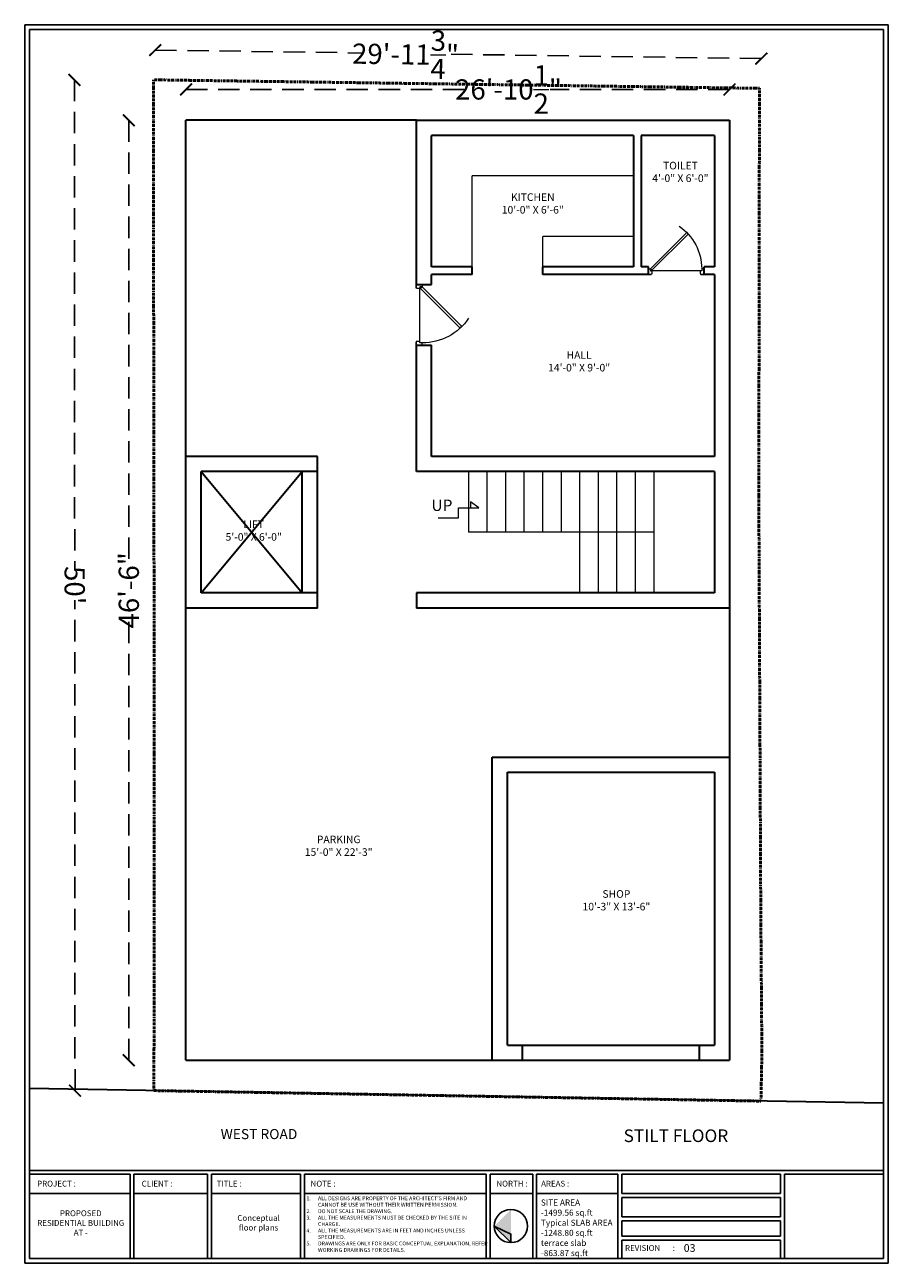
# Model space of a CAD drawing. Units: inches. Extents: x -16911 to -9621, y -48626 to -46270.
# Tile 1 of 20: x -16911 to -16399, y -47065 to -46330. Entities that reach past the tile are written whole.
import ezdxf

# ---------------------------------------------------------------- set-up
doc = ezdxf.new("R2010")
doc.units = ezdxf.units.IN
for name, pattern in [('DASHDOT', [1, 0.5, -0.25, 0, -0.25]), ('DASHED', [19.05, 12.7, -6.35]), ('DOT2', [3.175, 0, -3.175])]:
    doc.linetypes.add(name, pattern=pattern)
for name, color, linetype, lineweight in [('A-ANNO-DIMS', 2, 'Continuous', 13), ('A-ANNO-SYMB', 3, 'Continuous', 13), ('A-ANNO-TEXT', 7, 'Continuous', 18), ('A-ANNO-TTLB', 7, 'Continuous', 25), ('A-AREA-IDEN', 3, 'Continuous', 18), ('A-DOOR', 4, 'Continuous', 18), ('A-FLOR-STRS', 3, 'Continuous', 18), ('A-FURN', 8, 'Continuous', 13), ('A-WALL', 7, 'Continuous', 35), ('C-PROP', 6, 'DASHDOT', 50), ('DOOR', 143, 'Continuous', 9), ('STAIRCASE', 137, 'Continuous', 5)]:
    doc.layers.add(name, color=color, linetype=linetype, lineweight=lineweight)
doc.styles.get("Standard").update_dxf_attribs({"font": 'swissel.ttf'})
doc.styles.add('style9', font='swisscl.ttf', dxfattribs={"height": 12})
doc.dimstyles.new('Dim9', dxfattribs={"dimtxt": 10, "dimasz": 0.199219, "dimexe": 1, "dimexo": 0.5, "dimgap": 1, "dimtad": 0, "dimdec": 1, "dimzin": 0, "dimdsep": 46, "dimlunit": 4, "dimtxsty": 'style9', "dimblk": 'ARCHTICK', "dimcen": 0.09, "dimclrd": 256, "dimclrt": 256, "dimadec": 0, "dimazin": 0, "dimtfac": 1, "dimtdec": 1, "dimtix": 1, "dimtofl": 0, "dimtmove": 1, "dimatfit": 3, "dimfxl": 9, "dimtolj": 1, "dimtzin": 0, "dimlwd": -1, "dimarcsym": 0})

# ---------------------------------------------------------------- blocks, each defined once
blk = doc.blocks.new('_ArchTick')
at = {"color": 0, "linetype": 'ByBlock', "const_width": 0.15}
blk.add_lwpolyline([(-0.5, -0.5), (0.5, 0.5)], dxfattribs=at)
blk = doc.blocks.new('*D53')
at = {"layer": 'A-ANNO-DIMS', "color": 0, "linetype": 'DOT2', "lineweight": -2, "transparency": 16777216}
for p, q in [((-16834.02, -46345.34), (-16834, -46344.15)), ((-16474.35, -46350.39), (-16474.34, -46349.2))]:
    blk.add_line(p, q, dxfattribs=at)
at = {"layer": 'A-ANNO-DIMS', "color": 0, "linetype": 'DASHED', "lineweight": 25, "transparency": 16777216}
for p, q in [((-16834.01, -46345.15), (-16710.27, -46346.89)), ((-16474.35, -46350.2), (-16660.69, -46347.59))]:
    blk.add_line(p, q, dxfattribs=at)
at = {"layer": 'Defpoints', "color": 0, "transparency": 16777216}
for p in [(-16474.35, -46350.2), (-16834.21, -46359.07), (-16474.55, -46364.11)]:
    blk.add_point(p, dxfattribs=at)
at = {"layer": 'A-ANNO-DIMS', "color": 0, "lineweight": 25, "transparency": 16777216, "xscale": 7, "yscale": 7, "zscale": 7}
for p, rotation in [((-16834.01, -46345.15), 179.1963905603631), ((-16474.35, -46350.2), 359.196390560363)]:
    blk.add_blockref('_ArchTick', p, dxfattribs=dict(at, rotation=rotation))
at = {"layer": 'A-ANNO-DIMS', "color": 0, "transparency": 16777216, "insert": (-16685.49, -46347.68), "char_height": 12, "attachment_point": 5, "rotation": 359.19639, "style": 'style9'}
blk.add_mtext('\\A1;29\'-11{\\H1x;\\S3/4;}"', dxfattribs=at)
blk = doc.blocks.new('*D54')
at = {"layer": 'A-ANNO-DIMS', "color": 0, "linetype": 'DOT2', "lineweight": -2, "transparency": 16777216}
for p, q in [((-16881.81, -46362.82), (-16883, -46362.82)), ((-16881.44, -46962.82), (-16882.63, -46962.82))]:
    blk.add_line(p, q, dxfattribs=at)
at = {"layer": 'A-ANNO-DIMS', "color": 0, "linetype": 'DASHED', "lineweight": 25, "transparency": 16777216}
for p, q in [((-16882, -46362.82), (-16881.82, -46653.98)), ((-16881.63, -46962.82), (-16881.81, -46671.67))]:
    blk.add_line(p, q, dxfattribs=at)
at = {"layer": 'Defpoints', "color": 0, "transparency": 16777216}
for p in [(-16882, -46362.82), (-16863.18, -46362.81), (-16862.82, -46962.81)]:
    blk.add_point(p, dxfattribs=at)
at = {"layer": 'A-ANNO-DIMS', "color": 0, "lineweight": 25, "transparency": 16777216, "xscale": 7, "yscale": 7, "zscale": 7}
for p, rotation in [((-16882, -46362.82), 90.0346840750536), ((-16881.63, -46962.82), 270.0346840750536)]:
    blk.add_blockref('_ArchTick', p, dxfattribs=dict(at, rotation=rotation))
at = {"layer": 'A-ANNO-DIMS', "color": 0, "transparency": 16777216, "insert": (-16881.81, -46662.82), "char_height": 12, "attachment_point": 5, "rotation": 270.03468, "style": 'style9'}
blk.add_mtext("\\A1;50'", dxfattribs=at)
blk = doc.blocks.new('*D55')
at = {"layer": 'A-ANNO-DIMS', "color": 0, "linetype": 'DOT2', "lineweight": -2, "transparency": 16777216}
for p, q in [((-16815.78, -46368.33), (-16815.78, -46369.52)), ((-16493.23, -46368.33), (-16493.23, -46369.52))]:
    blk.add_line(p, q, dxfattribs=at)
at = {"layer": 'A-ANNO-DIMS', "color": 0, "linetype": 'DASHED', "lineweight": 25, "transparency": 16777216}
for p, q in [((-16815.78, -46368.52), (-16649, -46368.52)), ((-16493.23, -46368.52), (-16599.73, -46368.52))]:
    blk.add_line(p, q, dxfattribs=at)
at = {"layer": 'Defpoints', "color": 0, "transparency": 16777216}
for p in [(-16815.78, -46345.28), (-16493.23, -46345.28), (-16493.23, -46368.52)]:
    blk.add_point(p, dxfattribs=at)
at = {"layer": 'A-ANNO-DIMS', "color": 0, "lineweight": 25, "transparency": 16777216, "xscale": 7, "yscale": 7, "zscale": 7, "rotation": 180}
blk.add_blockref('_ArchTick', (-16815.78, -46368.52), dxfattribs=at)
at = {"layer": 'A-ANNO-DIMS', "color": 0, "lineweight": 25, "transparency": 16777216, "xscale": 7, "yscale": 7, "zscale": 7}
blk.add_blockref('_ArchTick', (-16493.23, -46368.52), dxfattribs=at)
at = {"layer": 'A-ANNO-DIMS', "color": 0, "transparency": 16777216, "insert": (-16624.37, -46368.52), "char_height": 12, "attachment_point": 5, "style": 'style9'}
blk.add_mtext('\\A1;26\'-10{\\H1x;\\S1/2;}"', dxfattribs=at)
blk = doc.blocks.new('*D56')
at = {"layer": 'A-ANNO-DIMS', "color": 0, "linetype": 'DOT2', "lineweight": -2, "transparency": 16777216}
for p, q in [((-16849.52, -46386.86), (-16850.71, -46386.86)), ((-16849.52, -46944.81), (-16850.71, -46944.81))]:
    blk.add_line(p, q, dxfattribs=at)
at = {"layer": 'A-ANNO-DIMS', "color": 0, "linetype": 'DASHED', "lineweight": 25, "transparency": 16777216}
for p, q in [((-16849.71, -46386.86), (-16849.71, -46648.2)), ((-16849.71, -46944.81), (-16849.71, -46683.47))]:
    blk.add_line(p, q, dxfattribs=at)
at = {"layer": 'Defpoints', "color": 0, "transparency": 16777216}
for p in [(-16815.78, -46386.86), (-16849.71, -46944.81), (-16815.78, -46944.81)]:
    blk.add_point(p, dxfattribs=at)
at = {"layer": 'A-ANNO-DIMS', "color": 0, "lineweight": 25, "transparency": 16777216, "xscale": 7, "yscale": 7, "zscale": 7}
for p, rotation in [((-16849.71, -46386.86), 90), ((-16849.71, -46944.81), 270)]:
    blk.add_blockref('_ArchTick', p, dxfattribs=dict(at, rotation=rotation))
at = {"layer": 'A-ANNO-DIMS', "color": 0, "transparency": 16777216, "insert": (-16849.71, -46665.83), "char_height": 12, "attachment_point": 5, "rotation": 90, "style": 'style9'}
blk.add_mtext('\\A1;46\'-6"', dxfattribs=at)
blk = doc.blocks.new('THYHYTJ')
at = {"layer": 'STAIRCASE', "ltscale": 10}
for p, q in [((-7981.18, -46346.18), (-7984.62, -46351.1)), ((-7981.18, -46358.18), (-7981.18, -46346.18)), ((-7984.62, -46351.1), (-7981.18, -46351.1)), ((-7975.18, -46358.18), (-7981.18, -46358.18)), ((-7975.18, -46370.18), (-7975.18, -46358.18))]:
    blk.add_line(p, q, dxfattribs=at)
blk = doc.blocks.new('A$C1C9D3E54')
at = {"layer": 'DOOR'}
blk.add_line((18676.53, 5780.72), (18710.53, 5780.72), dxfattribs=at)
blk.add_lwpolyline([(18685.01, 5806.62), (18710.47, 5781.16), (18711.53, 5782.22), (18686.07, 5807.68), (18685.01, 5806.62)], dxfattribs=at)
blk.add_lwpolyline([(18674.03, 5778.22), (18676.03, 5778.22), (18674.03, 5778.22), (18674.03, 5782.22), (18675.53, 5782.22), (18675.53, 5780.72), (18676.53, 5780.72), (18676.53, 5778.72), (18676.41, 5778.72), (18676.41, 5778.6, -0.414214), (18676.16, 5778.35), (18676.03, 5778.35), (18676.03, 5778.22)], format="xyb", dxfattribs=at)
blk.add_lwpolyline([(18713.03, 5782.22), (18711.53, 5782.22), (18711.53, 5780.72), (18710.53, 5780.72), (18710.53, 5778.72), (18710.66, 5778.72), (18710.66, 5778.6, 0.414214), (18710.91, 5778.35), (18711.03, 5778.35), (18711.03, 5778.22), (18713.03, 5778.22), (18711.03, 5778.22), (18713.03, 5778.22), (18713.03, 5782.22)], format="xyb", close=True, dxfattribs=at)
blk.add_arc((18711.53, 5782.22), 36, 124.03362, 180, dxfattribs=at)
blk = doc.blocks.new('TITLE-BLOCK-A3')
blk.add_hatch(color=256).paths.add_polyline_path([(-16032.81, -47043.2), (-16022.97, -47033.35), (-16022.97, -47053.05)])
for p, q in [((-16311.44, -47065.27), (-16311.44, -46330.13)), ((-16311.44, -46330.13), (-15799.07, -46330.13)), ((-16308.66, -47062.49), (-16308.66, -46332.91)), ((-16308.66, -46332.91), (-15801.86, -46332.91)), ((-15801.86, -46332.91), (-15801.86, -47062.49)), ((-15799.07, -46330.13), (-15799.07, -47065.27)), ((-15801.86, -47010.14), (-16308.66, -47010.14)), ((-16248.93, -47012.43), (-16308.66, -47012.43)), ((-16248.93, -47062.49), (-16248.93, -47012.43)), ((-16202.98, -47012.43), (-16246.63, -47012.43)), ((-16246.63, -47062.49), (-16246.63, -47012.43)), ((-16202.98, -47062.49), (-16202.98, -47012.43)), ((-16147.85, -47012.43), (-16200.68, -47012.43)), ((-16200.68, -47062.49), (-16200.68, -47012.43)), ((-16147.85, -47062.49), (-16147.85, -47012.43)), ((-16037.57, -47012.43), (-16145.55, -47012.43)), ((-16145.55, -47062.49), (-16145.55, -47012.43)), ((-16037.57, -47062.49), (-16037.57, -47012.43)), ((-16010.01, -47012.43), (-16035.28, -47012.43)), ((-16035.28, -47062.49), (-16035.28, -47012.43)), ((-16010.01, -47062.49), (-16010.01, -47012.43)), ((-15959.47, -47012.43), (-16007.71, -47012.43)), ((-16007.71, -47062.49), (-16007.71, -47012.43)), ((-15959.47, -47062.49), (-15959.47, -47012.43)), ((-15862.98, -47012.43), (-15957.17, -47012.43)), ((-15957.17, -47023.95), (-15957.17, -47012.43)), ((-15862.98, -47023.95), (-15862.98, -47012.43)), ((-15801.86, -47012.43), (-15860.68, -47012.43)), ((-15860.68, -47062.49), (-15860.68, -47012.43)), ((-16308.66, -47023.95), (-16248.93, -47023.95)), ((-16246.63, -47023.95), (-16202.98, -47023.95)), ((-16200.68, -47023.95), (-16147.85, -47023.95)), ((-16145.55, -47023.95), (-16037.57, -47023.95)), ((-16035.28, -47023.95), (-16010.01, -47023.95)), ((-16007.71, -47023.95), (-15959.47, -47023.95)), ((-15957.17, -47023.95), (-15862.98, -47023.95)), ((-15957.17, -47037.77), (-15957.17, -47026.25)), ((-15957.17, -47026.25), (-15862.98, -47026.25)), ((-15862.98, -47037.77), (-15862.98, -47026.25)), ((-15957.17, -47037.77), (-15862.98, -47037.77)), ((-15957.17, -47049.29), (-15957.17, -47040.07)), ((-15957.17, -47040.07), (-15862.98, -47040.07)), ((-15862.98, -47049.29), (-15862.98, -47040.07)), ((-15957.17, -47049.29), (-15862.98, -47049.29)), ((-15957.17, -47062.49), (-15957.17, -47051.59)), ((-15862.98, -47062.49), (-15862.98, -47051.59)), ((-15801.86, -47062.49), (-16308.66, -47062.49)), ((-15799.07, -47065.27), (-16311.44, -47065.27))]:
    blk.add_line(p, q)
blk.add_lwpolyline([(-16032.81, -47043.2), (-16022.97, -47047.92), (-16022.97, -47053.05), (-16032.81, -47043.2)])
blk.add_circle((-16022.97, -47043.2), 9.85)

msp = doc.modelspace()

# ---------------------------------------------------------------- linework, layer by layer
at = {"layer": 'A-ANNO-TTLB'}
msp.add_line((-16557.168, -47051.592), (-16462.978, -47051.592), dxfattribs=at)
at = {"layer": 'A-FLOR-STRS', "ltscale": 10}
for p, q in [((-16648.233, -46595.355), (-16648.233, -46631.355)), ((-16637.233, -46595.355), (-16637.233, -46631.355)), ((-16626.233, -46595.355), (-16626.233, -46631.355)), ((-16615.233, -46595.355), (-16615.233, -46631.355)), ((-16604.233, -46595.355), (-16604.233, -46631.355)), ((-16593.233, -46595.355), (-16593.233, -46631.355)), ((-16582.233, -46595.355), (-16582.233, -46667.355)), ((-16571.233, -46595.355), (-16571.233, -46667.355)), ((-16560.233, -46595.355), (-16560.233, -46667.355)), ((-16549.233, -46595.355), (-16549.233, -46667.355)), ((-16538.233, -46595.355), (-16538.233, -46667.355)), ((-16538.233, -46631.355), (-16648.233, -46631.355))]:
    msp.add_line(p, q, dxfattribs=at)
at = {"layer": 'A-FURN', "ltscale": 0.2}
for p, q in [((-16646.033, -46473.855), (-16646.033, -46419.855)), ((-16550.233, -46419.855), (-16646.033, -46419.855)), ((-16604.033, -46473.855), (-16604.033, -46455.855)), ((-16550.233, -46455.855), (-16604.033, -46455.855))]:
    msp.add_line(p, q, dxfattribs=at)
at = {"layer": 'A-WALL'}
for p, q in [((-16815.783, -46586.355), (-16815.783, -46386.855)), ((-16679.033, -46386.855), (-16815.783, -46386.855)), ((-16679.033, -46484.355), (-16679.033, -46386.855)), ((-16679.033, -46386.855), (-16493.233, -46386.855)), ((-16493.233, -46386.855), (-16493.233, -46676.355)), ((-16670.033, -46473.855), (-16670.033, -46395.855)), ((-16550.233, -46395.855), (-16670.033, -46395.855)), ((-16550.233, -46395.855), (-16550.233, -46473.855)), ((-16502.233, -46395.855), (-16545.733, -46395.855)), ((-16545.733, -46395.855), (-16545.733, -46473.855)), ((-16502.233, -46395.855), (-16502.233, -46473.855)), ((-16646.033, -46473.855), (-16670.033, -46473.855)), ((-16646.033, -46478.355), (-16646.033, -46473.855)), ((-16604.033, -46478.355), (-16604.033, -46473.855)), ((-16550.233, -46473.855), (-16604.033, -46473.855)), ((-16541.233, -46473.855), (-16545.733, -46473.855)), ((-16541.233, -46478.355), (-16541.233, -46473.855)), ((-16502.233, -46473.855), (-16508.233, -46473.855)), ((-16508.233, -46478.355), (-16508.233, -46473.855)), ((-16670.033, -46484.355), (-16670.033, -46478.355)), ((-16646.033, -46478.355), (-16670.033, -46478.355)), ((-16541.233, -46478.355), (-16604.033, -46478.355)), ((-16502.233, -46478.355), (-16508.233, -46478.355)), ((-16502.233, -46478.355), (-16502.233, -46586.355)), ((-16679.033, -46484.355), (-16670.033, -46484.355)), ((-16679.033, -46520.355), (-16670.033, -46520.355)), ((-16679.033, -46595.355), (-16679.033, -46520.355)), ((-16670.033, -46586.355), (-16670.033, -46520.355)), ((-16815.783, -46676.355), (-16815.783, -46586.355)), ((-16737.783, -46586.355), (-16815.783, -46586.355)), ((-16737.783, -46595.355), (-16737.783, -46586.355)), ((-16502.233, -46586.355), (-16670.033, -46586.355)), ((-16806.783, -46667.355), (-16806.783, -46595.355)), ((-16737.783, -46595.355), (-16806.783, -46595.355)), ((-16806.783, -46595.355), (-16746.783, -46667.355)), ((-16806.783, -46667.355), (-16746.783, -46595.355)), ((-16746.783, -46667.355), (-16746.783, -46595.355)), ((-16737.783, -46667.355), (-16737.783, -46595.355)), ((-16502.233, -46595.355), (-16679.033, -46595.355)), ((-16502.233, -46595.355), (-16502.233, -46667.355)), ((-16737.783, -46667.355), (-16806.783, -46667.355)), ((-16737.783, -46676.355), (-16737.783, -46667.355)), ((-16502.233, -46667.355), (-16679.033, -46667.355)), ((-16679.033, -46667.355), (-16679.033, -46676.355)), ((-16815.783, -46944.809), (-16815.783, -46676.355)), ((-16737.783, -46676.355), (-16815.783, -46676.355)), ((-16679.283, -46676.355), (-16679.283, -46676.355)), ((-16493.233, -46676.355), (-16679.033, -46676.355)), ((-16493.233, -46676.355), (-16493.233, -46764.809)), ((-16634.033, -46944.809), (-16634.033, -46764.809)), ((-16634.033, -46764.809), (-16493.233, -46764.809)), ((-16493.233, -46764.809), (-16493.233, -46944.809)), ((-16625.033, -46935.809), (-16625.033, -46773.809)), ((-16625.033, -46773.809), (-16502.233, -46773.809)), ((-16502.233, -46773.809), (-16502.233, -46935.809)), ((-16625.033, -46935.809), (-16616.033, -46935.809)), ((-16616.033, -46944.809), (-16616.033, -46935.809)), ((-16616.033, -46935.809), (-16511.233, -46935.809)), ((-16511.233, -46935.809), (-16511.233, -46944.809)), ((-16511.233, -46935.809), (-16502.233, -46935.809)), ((-16815.783, -46944.809), (-16634.033, -46944.809)), ((-16634.033, -46944.809), (-16616.033, -46944.809)), ((-16616.033, -46944.809), (-16511.233, -46944.809)), ((-16511.233, -46944.809), (-16493.233, -46944.809)), ((-16401.856, -46970.292), (-16908.658, -46961.533))]:
    msp.add_line(p, q, dxfattribs=at)
at = {"layer": 'C-PROP'}
msp.add_lwpolyline([(-16834.783, -46962.809), (-16474.601, -46969.035), (-16474.04, -46940.446), (-16474.703, -46855.606), (-16475.869, -46609.511), (-16475.483, -46367.855), (-16835.146, -46362.811), (-16834.608, -46762.955)], close=True, dxfattribs=at)

# ---------------------------------------------------------------- block references
at = {"layer": 'A-ANNO-SYMB', "rotation": 270.0000000000144}
msp.add_blockref('THYHYTJ', (29704.121, -54597.957), dxfattribs=at)
at = {"layer": 'A-ANNO-TTLB'}
msp.add_blockref('TITLE-BLOCK-A3', (-600, 0), dxfattribs=at)
at = {"layer": 'A-DOOR', "xscale": -0.8461538461538624, "yscale": 0.8461538461538624, "zscale": 0.8461538461538624}
msp.add_blockref('A$C1C9D3E54', (-707.38, -51367.622), dxfattribs=at)
at = {"layer": 'A-DOOR', "xscale": -0.9230769230769229, "yscale": 0.9230769230769229, "zscale": 0.9230769230769229, "rotation": 270}
msp.add_blockref('A$C1C9D3E54', (-22013.028, -63757.922), dxfattribs=at)

# ---------------------------------------------------------------- texts
at = {"layer": 'A-ANNO-TEXT'}
msp.add_text('UP', height=6.75, dxfattribs=at).set_placement((-16670.133, -46618.742))
at = {"layer": 'A-ANNO-TEXT', "ltscale": 10, "style": 'style9'}
for s, insert, char_height, width, attachment_point in [('\\A1;{\\fCentury Gothic|b0|i0|c0|p34;WEST ROAD}', (-16795.193, -46985.611), 6, 70.69764, 1), ('\\A1;{\\fCentury Gothic|b0|i0|c0|p34;STILT FLOOR}', (-16556.089, -46985.845), 7.5, 166.78033, 1), ('\\A1;\\pxql;{\\fCentury Gothic|b0|i0|c0|p34;PROJECT :}', (-16765.778, -47016.326), 3.44598, 138.32013, 3), ('\\A1;\\pxql;{\\fCentury Gothic|b0|i0|c0|p34;CLIENT :}', (-16687.669, -47016.326), 3.44598, 154.40134, 3), ('\\A1;\\pxql;{\\fCentury Gothic|b0|i0|c0|p34;TITLE :}', (-16659.24, -47016.326), 3.44598, 138.32013, 3), ('\\A1;\\pxql;{\\fCentury Gothic|b0|i0|c0|p34;NOTE :}', (-16573.671, -47016.326), 3.44598, 168.18525, 3), ('\\A1;\\pxql;{\\fCentury Gothic|b0|i0|c0|p34;NORTH :}', (-16463.4, -47016.326), 3.44598, 168.18525, 3), ('\\A1;\\pxql;{\\fCentury Gothic|b0|i0|c0|p34;AREAS :}', (-16466.711, -47016.326), 3.44598, 138.32013, 3), ("\\pxi-3,l4,ql,t4;{\\fArial|b0|i0|c0|p34;1.^IALL DESIGNS ARE PROPERTY OF THE ARCHITECT'S FIRM AND CANNOT BE USE WITHOUT THEIR WRITTEN PERMISSION.\\P2.^IDO NOT SCALE THE DRAWING.\\P3.^IALL THE MEASUREMENTS MUST BE CHECKED BY THE SITE IN CHARGE.\\P4.^IALL THE MEASUREMENTS ARE IN FEET AND INCHES UNLESS SPECIFIED.\\P5.^IDRAWINGS ARE ONLY FOR BASIC CONCEPTUAL EXPLANATION, REFER WORKING DRAWINGS FOR DETAILS.}", (-16636.219, -47025.582), 2.297317, 110.42201, 3), ('\\A1;\\pxqc;{\\fCentury Gothic|b0|i0|c0|p34;PROPOSED RESIDENTIAL BUILDING AT -}', (-16851.087, -47033.885), 3.44598, 54.24005, 3), ('\\A1;{\\fCentury Gothic|b0|i0|c0|p34;SITE AREA\\P-1499.56 sq.ft\\PTypical SLAB AREA \\P-1248.80 sq.ft\\Pterrace slab \\P-863.87 sq.ft }', (-16605.181, -47061.046), 3.6, 46.67019, 7), ('\\A1;\\pxqc;{\\fCentury Gothic|b0|i0|c0|p34;Conceptual\\Pfloor plans}', (-16758.709, -47036.671), 3.44598, 27.96068, 3), ('\\A1;\\pxql;{\\fCentury Gothic|b0|i0|c0|p34;REVISION       :     \\H1.33333x;03}', (-16416.939, -47053.939), 3.44598, 138.32013, 3)]:
    msp.add_mtext(s, dxfattribs=dict(at, insert=insert, char_height=char_height, width=width, attachment_point=attachment_point))
at = {"layer": 'A-AREA-IDEN', "ltscale": 10, "char_height": 4.5, "width": 42.823, "attachment_point": 1, "style": 'style9'}
for s, insert in [('\\A1;\\pxqc;{\\fCentury Gothic|b0|i0|c0|p34;TOILET\\P4\'-0" X 6\'-0"}', (-16543.805, -46411.463)), ('\\A1;\\pxqc;{\\fCentury Gothic|b0|i0|c0|p34;KITCHEN\\P10\'-0" X 6\'-6"}', (-16631.398, -46430.204)), ('\\A1;\\pxqc;{\\fCentury Gothic|b0|i0|c0|p34;HALL\\P14\'-0" X 9\'-0"}', (-16603.893, -46523.917)), ('\\A1;\\pxqc;{\\fCentury Gothic|b0|i0|c0|p34;LIFT\\P5\'-0" X 6\'-0"}', (-16797.007, -46624.39)), ('\\A1;\\pxqc;{\\fCentury Gothic|b0|i0|c0|p34;PARKING\\P15\'-0" X 22\'-3"}', (-16746.568, -46811.449)), ('\\A1;\\pxqc;{\\fCentury Gothic|b0|i0|c0|p34;SHOP\\P10\'-3" X 13\'-6"}', (-16581.778, -46843.832))]:
    msp.add_mtext(s, dxfattribs=dict(at, insert=insert))

# ---------------------------------------------------------------- dimensions: what is measured, and where the dimension line sits
at = {"layer": 'A-ANNO-DIMS'}
dim = msp.add_linear_dim(base=(-16474.352, -46350.199), p1=(-16834.21, -46359.069), p2=(-16474.547, -46364.114), angle=359.196391, dimstyle='Dim9', override={"dimtxt": 12, "dimasz": 7, "dimdec": 2, "dimclrd": 0, "dimclre": 0, "dimclrt": 0, "dimtdec": 2, "dimfxl": 0.1875, "dimfxlon": 1, "dimlwd": 25, "dimarcsym": 2}, dxfattribs=at)
dim.commit()
dim.dimension.update_dxf_attribs({"geometry": '*D53', "text_midpoint": (-16685.488, -46347.677), "dimtype": 161})
dim = msp.add_linear_dim(base=(-16493.233, -46368.516), p1=(-16815.783, -46345.28), p2=(-16493.233, -46345.28), dimstyle='Dim9', override={"dimtxt": 12, "dimasz": 7, "dimdec": 2, "dimclrd": 0, "dimclre": 0, "dimclrt": 0, "dimtdec": 2, "dimfxl": 0.1875, "dimfxlon": 1, "dimlwd": 25, "dimarcsym": 2}, dxfattribs=at)
dim.commit()
dim.dimension.update_dxf_attribs({"geometry": '*D55', "text_midpoint": (-16624.367, -46368.516), "dimtype": 160})
dim = msp.add_aligned_dim(p1=(-16862.815, -46962.809), p2=(-16863.178, -46362.811), distance=18.817, dimstyle='Dim9', override={"dimtxt": 12, "dimasz": 7, "dimdec": 2, "dimclrd": 0, "dimclre": 0, "dimclrt": 0, "dimtdec": 2, "dimfxl": 0.1875, "dimfxlon": 1, "dimlwd": 25, "dimarcsym": 2}, dxfattribs=at)
dim.commit()
dim.dimension.update_dxf_attribs({"geometry": '*D54', "text_midpoint": (-16881.814, -46662.821)})
dim = msp.add_linear_dim(base=(-16849.711, -46944.809), p1=(-16815.783, -46386.855), p2=(-16815.783, -46944.809), angle=90, dimstyle='Dim9', override={"dimtxt": 12, "dimasz": 7, "dimdec": 2, "dimclrd": 0, "dimclre": 0, "dimclrt": 0, "dimtdec": 2, "dimfxl": 0.1875, "dimfxlon": 1, "dimlwd": 25, "dimarcsym": 2}, dxfattribs=at)
dim.commit()
dim.dimension.update_dxf_attribs({"geometry": '*D56', "text_midpoint": (-16849.711, -46665.832)})

doc.saveas('drawing.dxf')
